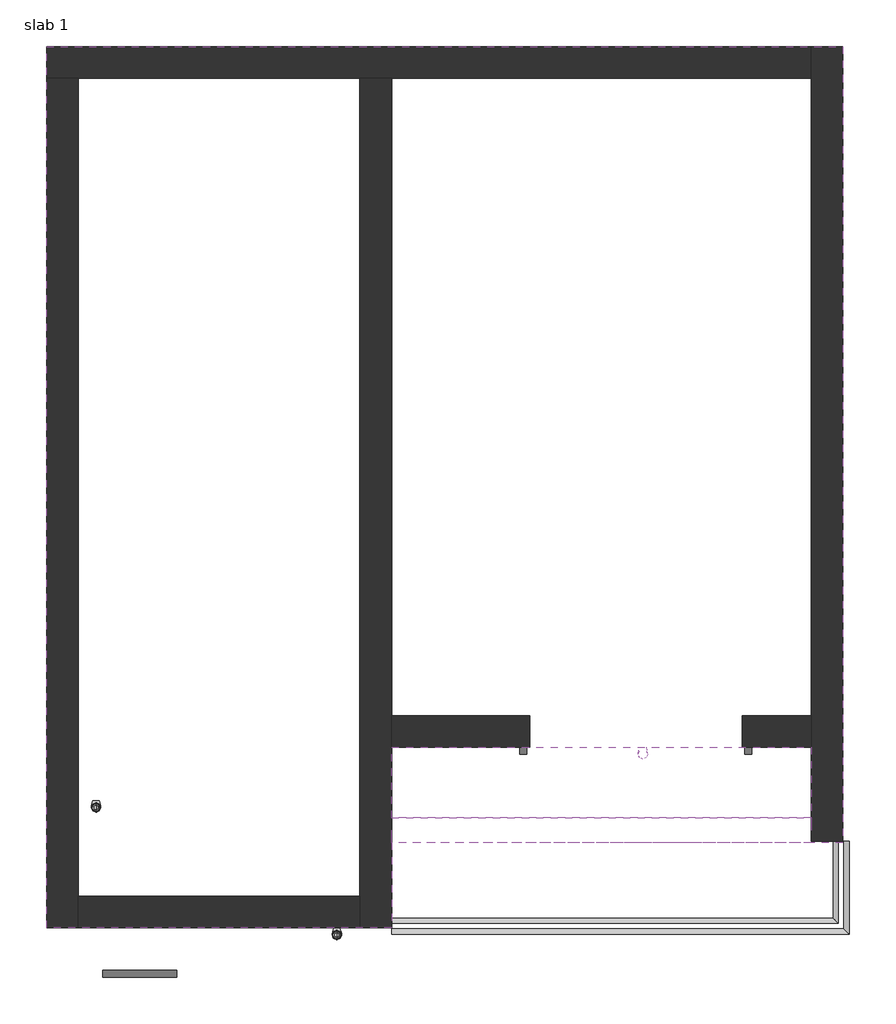
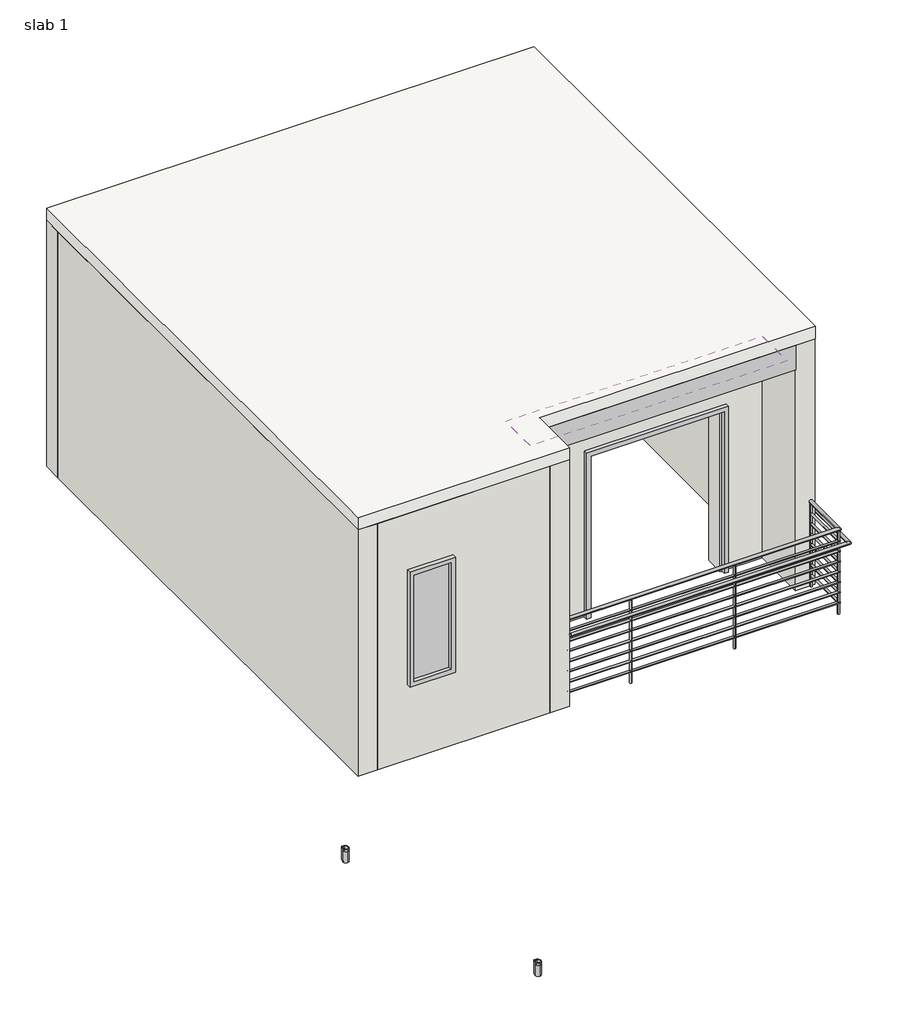
# One storey: 6 walls, 3 light fixtures, 3 proxies, 1 covering, 1 railing, 1 slab.
"""IFC4 building model written with IfcOpenShell, lengths in millimetres."""

from ifc_helpers import new_model, si_unit, point, frame, frame_2d, origin, place, context, project, spatial, polyline, circle_curve, ellipse_curve, trimmed, segment, composite_curve, outline, extrude, faceted_brep, transform, mapped, element, save
from ifc_brep_helpers import plane_surface, cylinder_surface, advanced_brep
from components import generic_models_1_generic_models_1_53319598, generic_models_3_generic_models_3_c6119d6a, generic_models_4_generic_models_4_090447d9, light_fixture_d13112ec

model = new_model("IFC4")

# Units and contexts
model_context = context("Model", 3, world=origin())
ifc_project = project(units=[si_unit("LENGTHUNIT", "METRE", prefix="MILLI")], contexts=[model_context])

# Site, building, storey
site = spatial("IfcSite", under=ifc_project)
building = spatial("IfcBuilding", under=site)
storey = spatial("IfcBuildingStorey", under=building, Name="slab 1", Elevation=3200.4)

# Proxies
placement = place(None, origin())
generic_models_1_generic_models_1_shape = generic_models_1_generic_models_1_53319598(model_context)
element("IfcBuildingElementProxy", 1, Name="Generic Models 1 : Generic Models 1", ObjectType="Generic Models 1 : Generic Models 1", at=placement, inside=storey, context=model_context, shape_type="MappedRepresentation", body=[
    mapped(generic_models_1_generic_models_1_shape, transform((0.0, 0.0, 0.0), x_axis=(1.0, 0.0, 0.0), y_axis=(0.0, 1.0, 0.0), z_axis=(0.0, 0.0, 1.0))),
])
generic_models_3_generic_models_3_shape = generic_models_3_generic_models_3_c6119d6a(model_context)
element("IfcBuildingElementProxy", 2, Name="Generic Models 3 : Generic Models 3", ObjectType="Generic Models 3 : Generic Models 3", at=placement, inside=storey, context=model_context, shape_type="MappedRepresentation", body=[
    mapped(generic_models_3_generic_models_3_shape, transform((0.0, 0.0, 0.0), x_axis=(1.0, 0.0, 0.0), y_axis=(0.0, 1.0, 0.0), z_axis=(0.0, 0.0, 1.0))),
])
generic_models_4_generic_models_4_shape = generic_models_4_generic_models_4_090447d9(model_context)
element("IfcBuildingElementProxy", 3, Name="Generic Models 4 : Generic Models 4", ObjectType="Generic Models 4 : Generic Models 4", at=placement, inside=storey, context=model_context, shape_type="MappedRepresentation", body=[
    mapped(generic_models_4_generic_models_4_shape, transform((0.0, 0.0, 0.0), x_axis=(1.0, 0.0, 0.0), y_axis=(0.0, 1.0, 0.0), z_axis=(0.0, 0.0, 1.0))),
])

# Covering
element("IfcCovering", 4, ObjectType="2' x 4' ACT System", at=placement, inside=storey, context=model_context, shape_type="SweptSolid", body=[
    extrude(outline(polyline([(-4601.1678816, 2126.5115792), (-7611.0678816, 2126.5115792), (-7611.0678816, 2631.9030358), (-4601.1678816, 2631.9030358), (-4601.1678816, 2126.5115792)])), frame((0.0, 0.0, 5943.6), z_axis=(0.0, 0.0, 1.0), x_axis=(1.0, 0.0, 0.0)), (0.0, 0.0, 1.0), 57.15),
])

# Light fixtures
light_fixture_shape = light_fixture_d13112ec(model_context)
element("IfcLightFixture", 5, at=placement, inside=storey, context=model_context, shape_type="MappedRepresentation", body=[
    mapped(light_fixture_shape, transform((-9731.9678816, 2250.9030358, 1580.2048365), x_axis=(1.0, 0.0, 0.0), y_axis=(0.0, 1.0, 0.0), z_axis=(0.0, 0.0, 1.0))),
])
element("IfcLightFixture", 6, at=placement, inside=storey, context=model_context, shape_type="MappedRepresentation", body=[
    mapped(light_fixture_shape, transform((-8004.7678816, 1336.5030358, 122.3083), x_axis=(1.0, 0.0, 0.0), y_axis=(0.0, 1.0, 0.0), z_axis=(0.0, 0.0, 1.0))),
])
element("IfcLightFixture", 7, at=placement, inside=storey, context=model_context, shape_type="MappedRepresentation", body=[
    mapped(light_fixture_shape, transform((-5808.000689, 2631.9030358, 5856.5439655), x_axis=(1.0, 0.0, 0.0), y_axis=(0.0, 1.0, 0.0), z_axis=(0.0, 0.0, 1.0))),
])

# Railing
element("IfcRailing", 8, ObjectType="Guardrail - Pipe", at=placement, inside=storey, context=model_context, shape_type="SolidModel", body=[
    advanced_brep(
    [(-4366.2178816, 1958.8030358, 4095.75), (-4328.1178816, 1958.8030358, 4095.75), (-4366.2178816, 1330.1530358, 4095.75), (-4328.1178816, 1292.0530358, 4095.75), (-7611.0678816, 1330.1530358, 4095.75), (-7611.0678816, 1292.0530358, 4095.75)],
    [
        (0, 1, circle_curve(frame((-4347.1678816, 1958.8030358, 4095.75), z_axis=(0.0, 1.0, 0.0), x_axis=(1.0, 0.0, 0.0)), 19.05)),
        (1, 0, circle_curve(frame((-4347.1678816, 1958.8030358, 4095.75), z_axis=(0.0, 1.0, 0.0), x_axis=(1.0, 0.0, 0.0)), 19.05)),
        (0, 2),
        (2, 3, ellipse_curve(frame((-4347.1678816, 1311.1030358, 4095.75), z_axis=(0.7071067811865487, 0.7071067811865464, 0.0), x_axis=(-0.7071067811865464, 0.7071067811865487, 0.0)), 26.9407684, 19.05)),
        (3, 1),
        (3, 2, ellipse_curve(frame((-4347.1678816, 1311.1030358, 4095.75), z_axis=(0.7071067811865487, 0.7071067811865464, 0.0), x_axis=(-0.7071067811865464, 0.7071067811865487, 0.0)), 26.9407684, 19.05)),
        (4, 5, circle_curve(frame((-7611.0678816, 1311.1030358, 4095.75), z_axis=(-1.0, 0.0, 0.0), x_axis=(0.0, -1.0, 0.0)), 19.05)),
        (5, 4, circle_curve(frame((-7611.0678816, 1311.1030358, 4095.75), z_axis=(-1.0, 0.0, 0.0), x_axis=(0.0, -1.0, 0.0)), 19.05)),
        (2, 4),
        (5, 3),
    ],
    [
        plane_surface(frame((-4347.1678816, 1958.8030358, 4114.8), z_axis=(0.0, 1.0, 0.0), x_axis=(0.0, 0.0, -1.0))),
        cylinder_surface(frame((-4347.1678816, 1958.8030358, 4095.75), z_axis=(0.0, 1.0, 0.0), x_axis=(1.0, 0.0, 0.0)), 19.05),
        plane_surface(frame((-7611.0678816, 1311.1030358, 4114.8), z_axis=(-1.0, 0.0, 0.0), x_axis=(0.0, -1.0, 0.0))),
        cylinder_surface(frame((-4347.1678816, 1311.1030358, 4095.75), z_axis=(1.0, 0.0, 0.0), x_axis=(0.0, -1.0, 0.0)), 19.05),
    ],
    [
        (0, [[1, 2]]),
        (1, [[-1, 3, 4, 5]]),
        (1, [[-2, -5, 6, -3]]),
        (2, [[7, 8]]),
        (3, [[-4, 9, -8, 10]]),
        (3, [[-6, -10, -7, -9]]),
    ],
),
    advanced_brep(
    [(-4442.4178816, 1958.8030358, 4248.15), (-4404.3178816, 1958.8030358, 4248.15), (-7611.0678816, 1406.3530358, 4248.15), (-7611.0678816, 1368.2530358, 4248.15), (-4442.4178816, 1406.3530358, 4248.15), (-4404.3178816, 1368.2530358, 4248.15)],
    [
        (0, 1, circle_curve(frame((-4423.3678816, 1958.8030358, 4248.15), z_axis=(0.0, 1.0, 0.0), x_axis=(1.0, 0.0, 0.0)), 19.05)),
        (1, 0, circle_curve(frame((-4423.3678816, 1958.8030358, 4248.15), z_axis=(0.0, 1.0, 0.0), x_axis=(1.0, 0.0, 0.0)), 19.05)),
        (2, 3, circle_curve(frame((-7611.0678816, 1387.3030358, 4248.15), z_axis=(-1.0, 0.0, 0.0), x_axis=(0.0, -1.0, 0.0)), 19.05)),
        (3, 2, circle_curve(frame((-7611.0678816, 1387.3030358, 4248.15), z_axis=(-1.0, 0.0, 0.0), x_axis=(0.0, -1.0, 0.0)), 19.05)),
        (0, 4),
        (4, 5, ellipse_curve(frame((-4423.3678816, 1387.3030358, 4248.15), z_axis=(0.7071067811865487, 0.7071067811865464, 0.0), x_axis=(-0.7071067811865464, 0.7071067811865487, 0.0)), 26.9407684, 19.05)),
        (5, 1),
        (5, 4, ellipse_curve(frame((-4423.3678816, 1387.3030358, 4248.15), z_axis=(0.7071067811865487, 0.7071067811865464, 0.0), x_axis=(-0.7071067811865464, 0.7071067811865487, 0.0)), 26.9407684, 19.05)),
        (4, 2),
        (3, 5),
    ],
    [
        plane_surface(frame((-4423.3678816, 1958.8030358, 4267.2), z_axis=(0.0, 1.0, 0.0), x_axis=(0.0, 0.0, -1.0))),
        plane_surface(frame((-7611.0678816, 1387.3030358, 4267.2), z_axis=(-1.0, 0.0, 0.0), x_axis=(0.0, -1.0, 0.0))),
        cylinder_surface(frame((-4423.3678816, 1958.8030358, 4248.15), z_axis=(0.0, 1.0, 0.0), x_axis=(1.0, 0.0, 0.0)), 19.05),
        cylinder_surface(frame((-4423.3678816, 1387.3030358, 4248.15), z_axis=(1.0, 0.0, 0.0), x_axis=(0.0, -1.0, 0.0)), 19.05),
    ],
    [
        (0, [[1, 2]]),
        (1, [[3, 4]]),
        (2, [[-1, 5, 6, 7]]),
        (2, [[-2, -7, 8, -5]]),
        (3, [[-6, 9, -4, 10]]),
        (3, [[-8, -10, -3, -9]]),
    ],
),
    advanced_brep(
    [(-4410.6678816, 1958.8030358, 4102.1), (-4436.0678816, 1958.8030358, 4102.1), (-7611.0678816, 1374.6030358, 4102.1), (-7611.0678816, 1400.0030358, 4102.1), (-4410.6678816, 1374.6030358, 4102.1), (-4436.0678816, 1400.0030358, 4102.1)],
    [
        (0, 1, circle_curve(frame((-4423.3678816, 1958.8030358, 4102.1), z_axis=(0.0, 1.0, 0.0), x_axis=(-1.0, 0.0, 0.0)), 12.7)),
        (1, 0, circle_curve(frame((-4423.3678816, 1958.8030358, 4102.1), z_axis=(0.0, 1.0, 0.0), x_axis=(-1.0, 0.0, 0.0)), 12.7)),
        (2, 3, circle_curve(frame((-7611.0678816, 1387.3030358, 4102.1), z_axis=(-1.0, 0.0, 0.0), x_axis=(0.0, 1.0, 0.0)), 12.7)),
        (3, 2, circle_curve(frame((-7611.0678816, 1387.3030358, 4102.1), z_axis=(-1.0, 0.0, 0.0), x_axis=(0.0, 1.0, 0.0)), 12.7)),
        (0, 4),
        (4, 5, ellipse_curve(frame((-4423.3678816, 1387.3030358, 4102.1), z_axis=(0.7071067811865487, 0.7071067811865464, 0.0), x_axis=(-0.7071067811865464, 0.7071067811865487, 0.0)), 17.9605122, 12.7)),
        (5, 1),
        (5, 4, ellipse_curve(frame((-4423.3678816, 1387.3030358, 4102.1), z_axis=(0.7071067811865487, 0.7071067811865464, 0.0), x_axis=(-0.7071067811865464, 0.7071067811865487, 0.0)), 17.9605122, 12.7)),
        (4, 2),
        (3, 5),
    ],
    [
        plane_surface(frame((-4423.3678816, 1958.8030358, 4114.8), z_axis=(0.0, 1.0, 0.0), x_axis=(0.0, 0.0, -1.0))),
        plane_surface(frame((-7611.0678816, 1387.3030358, 4114.8), z_axis=(-1.0, 0.0, 0.0), x_axis=(0.0, -1.0, 0.0))),
        cylinder_surface(frame((-4423.3678816, 1958.8030358, 4102.1), z_axis=(0.0, 1.0, 0.0), x_axis=(-1.0, 0.0, 0.0)), 12.7),
        cylinder_surface(frame((-4423.3678816, 1387.3030358, 4102.1), z_axis=(1.0, 0.0, 0.0), x_axis=(0.0, 1.0, 0.0)), 12.7),
    ],
    [
        (0, [[1, 2]]),
        (1, [[3, 4]]),
        (2, [[-1, 5, 6, 7]]),
        (2, [[-2, -7, 8, -5]]),
        (3, [[-6, 9, -4, 10]]),
        (3, [[-8, -10, -3, -9]]),
    ],
),
    advanced_brep(
    [(-4410.6678816, 1958.8030358, 3975.1), (-4436.0678816, 1958.8030358, 3975.1), (-7611.0678816, 1374.6030358, 3975.1), (-7611.0678816, 1400.0030358, 3975.1), (-4410.6678816, 1374.6030358, 3975.1), (-4436.0678816, 1400.0030358, 3975.1)],
    [
        (0, 1, circle_curve(frame((-4423.3678816, 1958.8030358, 3975.1), z_axis=(0.0, 1.0, 0.0), x_axis=(-1.0, 0.0, 0.0)), 12.7)),
        (1, 0, circle_curve(frame((-4423.3678816, 1958.8030358, 3975.1), z_axis=(0.0, 1.0, 0.0), x_axis=(-1.0, 0.0, 0.0)), 12.7)),
        (2, 3, circle_curve(frame((-7611.0678816, 1387.3030358, 3975.1), z_axis=(-1.0, 0.0, 0.0), x_axis=(0.0, 1.0, 0.0)), 12.7)),
        (3, 2, circle_curve(frame((-7611.0678816, 1387.3030358, 3975.1), z_axis=(-1.0, 0.0, 0.0), x_axis=(0.0, 1.0, 0.0)), 12.7)),
        (0, 4),
        (4, 5, ellipse_curve(frame((-4423.3678816, 1387.3030358, 3975.1), z_axis=(0.7071067811865487, 0.7071067811865464, 0.0), x_axis=(-0.7071067811865464, 0.7071067811865487, 0.0)), 17.9605122, 12.7)),
        (5, 1),
        (5, 4, ellipse_curve(frame((-4423.3678816, 1387.3030358, 3975.1), z_axis=(0.7071067811865487, 0.7071067811865464, 0.0), x_axis=(-0.7071067811865464, 0.7071067811865487, 0.0)), 17.9605122, 12.7)),
        (4, 2),
        (3, 5),
    ],
    [
        plane_surface(frame((-4423.3678816, 1958.8030358, 3987.8), z_axis=(0.0, 1.0, 0.0), x_axis=(0.0, 0.0, -1.0))),
        plane_surface(frame((-7611.0678816, 1387.3030358, 3987.8), z_axis=(-1.0, 0.0, 0.0), x_axis=(0.0, -1.0, 0.0))),
        cylinder_surface(frame((-4423.3678816, 1958.8030358, 3975.1), z_axis=(0.0, 1.0, 0.0), x_axis=(-1.0, 0.0, 0.0)), 12.7),
        cylinder_surface(frame((-4423.3678816, 1387.3030358, 3975.1), z_axis=(1.0, 0.0, 0.0), x_axis=(0.0, 1.0, 0.0)), 12.7),
    ],
    [
        (0, [[1, 2]]),
        (1, [[3, 4]]),
        (2, [[-1, 5, 6, 7]]),
        (2, [[-2, -7, 8, -5]]),
        (3, [[-6, 9, -4, 10]]),
        (3, [[-8, -10, -3, -9]]),
    ],
),
    advanced_brep(
    [(-4410.6678816, 1958.8030358, 3848.1), (-4436.0678816, 1958.8030358, 3848.1), (-4410.6678816, 1374.6030358, 3848.1), (-4436.0678816, 1400.0030358, 3848.1), (-7611.0678816, 1374.6030358, 3848.1), (-7611.0678816, 1400.0030358, 3848.1)],
    [
        (0, 1, circle_curve(frame((-4423.3678816, 1958.8030358, 3848.1), z_axis=(0.0, 1.0, 0.0), x_axis=(-1.0, 0.0, 0.0)), 12.7)),
        (1, 0, circle_curve(frame((-4423.3678816, 1958.8030358, 3848.1), z_axis=(0.0, 1.0, 0.0), x_axis=(-1.0, 0.0, 0.0)), 12.7)),
        (0, 2),
        (2, 3, ellipse_curve(frame((-4423.3678816, 1387.3030358, 3848.1), z_axis=(0.7071067811865487, 0.7071067811865464, 0.0), x_axis=(-0.7071067811865464, 0.7071067811865487, 0.0)), 17.9605122, 12.7)),
        (3, 1),
        (3, 2, ellipse_curve(frame((-4423.3678816, 1387.3030358, 3848.1), z_axis=(0.7071067811865487, 0.7071067811865464, 0.0), x_axis=(-0.7071067811865464, 0.7071067811865487, 0.0)), 17.9605122, 12.7)),
        (4, 5, circle_curve(frame((-7611.0678816, 1387.3030358, 3848.1), z_axis=(-1.0, 0.0, 0.0), x_axis=(0.0, 1.0, 0.0)), 12.7)),
        (5, 4, circle_curve(frame((-7611.0678816, 1387.3030358, 3848.1), z_axis=(-1.0, 0.0, 0.0), x_axis=(0.0, 1.0, 0.0)), 12.7)),
        (2, 4),
        (5, 3),
    ],
    [
        plane_surface(frame((-4423.3678816, 1958.8030358, 3860.8), z_axis=(0.0, 1.0, 0.0), x_axis=(0.0, 0.0, -1.0))),
        cylinder_surface(frame((-4423.3678816, 1958.8030358, 3848.1), z_axis=(0.0, 1.0, 0.0), x_axis=(-1.0, 0.0, 0.0)), 12.7),
        plane_surface(frame((-7611.0678816, 1387.3030358, 3860.8), z_axis=(-1.0, 0.0, 0.0), x_axis=(0.0, -1.0, 0.0))),
        cylinder_surface(frame((-4423.3678816, 1387.3030358, 3848.1), z_axis=(1.0, 0.0, 0.0), x_axis=(0.0, 1.0, 0.0)), 12.7),
    ],
    [
        (0, [[1, 2]]),
        (1, [[-1, 3, 4, 5]]),
        (1, [[-2, -5, 6, -3]]),
        (2, [[7, 8]]),
        (3, [[-4, 9, -8, 10]]),
        (3, [[-6, -10, -7, -9]]),
    ],
),
    advanced_brep(
    [(-4410.6678816, 1958.8030358, 3721.1), (-4436.0678816, 1958.8030358, 3721.1), (-4410.6678816, 1374.6030358, 3721.1), (-4436.0678816, 1400.0030358, 3721.1), (-7611.0678816, 1374.6030358, 3721.1), (-7611.0678816, 1400.0030358, 3721.1)],
    [
        (0, 1, circle_curve(frame((-4423.3678816, 1958.8030358, 3721.1), z_axis=(0.0, 1.0, 0.0), x_axis=(-1.0, 0.0, 0.0)), 12.7)),
        (1, 0, circle_curve(frame((-4423.3678816, 1958.8030358, 3721.1), z_axis=(0.0, 1.0, 0.0), x_axis=(-1.0, 0.0, 0.0)), 12.7)),
        (0, 2),
        (2, 3, ellipse_curve(frame((-4423.3678816, 1387.3030358, 3721.1), z_axis=(0.7071067811865487, 0.7071067811865464, 0.0), x_axis=(-0.7071067811865464, 0.7071067811865487, 0.0)), 17.9605122, 12.7)),
        (3, 1),
        (3, 2, ellipse_curve(frame((-4423.3678816, 1387.3030358, 3721.1), z_axis=(0.7071067811865487, 0.7071067811865464, 0.0), x_axis=(-0.7071067811865464, 0.7071067811865487, 0.0)), 17.9605122, 12.7)),
        (4, 5, circle_curve(frame((-7611.0678816, 1387.3030358, 3721.1), z_axis=(-1.0, 0.0, 0.0), x_axis=(0.0, 1.0, 0.0)), 12.7)),
        (5, 4, circle_curve(frame((-7611.0678816, 1387.3030358, 3721.1), z_axis=(-1.0, 0.0, 0.0), x_axis=(0.0, 1.0, 0.0)), 12.7)),
        (2, 4),
        (5, 3),
    ],
    [
        plane_surface(frame((-4423.3678816, 1958.8030358, 3733.8), z_axis=(0.0, 1.0, 0.0), x_axis=(0.0, 0.0, -1.0))),
        cylinder_surface(frame((-4423.3678816, 1958.8030358, 3721.1), z_axis=(0.0, 1.0, 0.0), x_axis=(-1.0, 0.0, 0.0)), 12.7),
        plane_surface(frame((-7611.0678816, 1387.3030358, 3733.8), z_axis=(-1.0, 0.0, 0.0), x_axis=(0.0, -1.0, 0.0))),
        cylinder_surface(frame((-4423.3678816, 1387.3030358, 3721.1), z_axis=(1.0, 0.0, 0.0), x_axis=(0.0, 1.0, 0.0)), 12.7),
    ],
    [
        (0, [[1, 2]]),
        (1, [[-1, 3, 4, 5]]),
        (1, [[-2, -5, 6, -3]]),
        (2, [[7, 8]]),
        (3, [[-4, 9, -8, 10]]),
        (3, [[-6, -10, -7, -9]]),
    ],
),
    advanced_brep(
    [(-4410.6678816, 1958.8030358, 3594.1), (-4436.0678816, 1958.8030358, 3594.1), (-4410.6678816, 1374.6030358, 3594.1), (-4436.0678816, 1400.0030358, 3594.1), (-7611.0678816, 1374.6030358, 3594.1), (-7611.0678816, 1400.0030358, 3594.1)],
    [
        (0, 1, circle_curve(frame((-4423.3678816, 1958.8030358, 3594.1), z_axis=(0.0, 1.0, 0.0), x_axis=(-1.0, 0.0, 0.0)), 12.7)),
        (1, 0, circle_curve(frame((-4423.3678816, 1958.8030358, 3594.1), z_axis=(0.0, 1.0, 0.0), x_axis=(-1.0, 0.0, 0.0)), 12.7)),
        (0, 2),
        (2, 3, ellipse_curve(frame((-4423.3678816, 1387.3030358, 3594.1), z_axis=(0.7071067811865487, 0.7071067811865464, 0.0), x_axis=(-0.7071067811865464, 0.7071067811865487, 0.0)), 17.9605122, 12.7)),
        (3, 1),
        (3, 2, ellipse_curve(frame((-4423.3678816, 1387.3030358, 3594.1), z_axis=(0.7071067811865487, 0.7071067811865464, 0.0), x_axis=(-0.7071067811865464, 0.7071067811865487, 0.0)), 17.9605122, 12.7)),
        (4, 5, circle_curve(frame((-7611.0678816, 1387.3030358, 3594.1), z_axis=(-1.0, 0.0, 0.0), x_axis=(0.0, 1.0, 0.0)), 12.7)),
        (5, 4, circle_curve(frame((-7611.0678816, 1387.3030358, 3594.1), z_axis=(-1.0, 0.0, 0.0), x_axis=(0.0, 1.0, 0.0)), 12.7)),
        (2, 4),
        (5, 3),
    ],
    [
        plane_surface(frame((-4423.3678816, 1958.8030358, 3606.8), z_axis=(0.0, 1.0, 0.0), x_axis=(0.0, 0.0, -1.0))),
        cylinder_surface(frame((-4423.3678816, 1958.8030358, 3594.1), z_axis=(0.0, 1.0, 0.0), x_axis=(-1.0, 0.0, 0.0)), 12.7),
        plane_surface(frame((-7611.0678816, 1387.3030358, 3606.8), z_axis=(-1.0, 0.0, 0.0), x_axis=(0.0, -1.0, 0.0))),
        cylinder_surface(frame((-4423.3678816, 1387.3030358, 3594.1), z_axis=(1.0, 0.0, 0.0), x_axis=(0.0, 1.0, 0.0)), 12.7),
    ],
    [
        (0, [[1, 2]]),
        (1, [[-1, 3, 4, 5]]),
        (1, [[-2, -5, 6, -3]]),
        (2, [[7, 8]]),
        (3, [[-4, 9, -8, 10]]),
        (3, [[-6, -10, -7, -9]]),
    ],
),
    advanced_brep(
    [(-4410.6678816, 1958.8030358, 3467.1), (-4436.0678816, 1958.8030358, 3467.1), (-4410.6678816, 1374.6030358, 3467.1), (-4436.0678816, 1400.0030358, 3467.1), (-7611.0678816, 1374.6030358, 3467.1), (-7611.0678816, 1400.0030358, 3467.1)],
    [
        (0, 1, circle_curve(frame((-4423.3678816, 1958.8030358, 3467.1), z_axis=(0.0, 1.0, 0.0), x_axis=(-1.0, 0.0, 0.0)), 12.7)),
        (1, 0, circle_curve(frame((-4423.3678816, 1958.8030358, 3467.1), z_axis=(0.0, 1.0, 0.0), x_axis=(-1.0, 0.0, 0.0)), 12.7)),
        (0, 2),
        (2, 3, ellipse_curve(frame((-4423.3678816, 1387.3030358, 3467.1), z_axis=(0.7071067811865487, 0.7071067811865464, 0.0), x_axis=(-0.7071067811865464, 0.7071067811865487, 0.0)), 17.9605122, 12.7)),
        (3, 1),
        (3, 2, ellipse_curve(frame((-4423.3678816, 1387.3030358, 3467.1), z_axis=(0.7071067811865487, 0.7071067811865464, 0.0), x_axis=(-0.7071067811865464, 0.7071067811865487, 0.0)), 17.9605122, 12.7)),
        (4, 5, circle_curve(frame((-7611.0678816, 1387.3030358, 3467.1), z_axis=(-1.0, 0.0, 0.0), x_axis=(0.0, 1.0, 0.0)), 12.7)),
        (5, 4, circle_curve(frame((-7611.0678816, 1387.3030358, 3467.1), z_axis=(-1.0, 0.0, 0.0), x_axis=(0.0, 1.0, 0.0)), 12.7)),
        (2, 4),
        (5, 3),
    ],
    [
        plane_surface(frame((-4423.3678816, 1958.8030358, 3479.8), z_axis=(0.0, 1.0, 0.0), x_axis=(0.0, 0.0, -1.0))),
        cylinder_surface(frame((-4423.3678816, 1958.8030358, 3467.1), z_axis=(0.0, 1.0, 0.0), x_axis=(-1.0, 0.0, 0.0)), 12.7),
        plane_surface(frame((-7611.0678816, 1387.3030358, 3479.8), z_axis=(-1.0, 0.0, 0.0), x_axis=(0.0, -1.0, 0.0))),
        cylinder_surface(frame((-4423.3678816, 1387.3030358, 3467.1), z_axis=(1.0, 0.0, 0.0), x_axis=(0.0, 1.0, 0.0)), 12.7),
    ],
    [
        (0, [[1, 2]]),
        (1, [[-1, 3, 4, 5]]),
        (1, [[-2, -5, 6, -3]]),
        (2, [[7, 8]]),
        (3, [[-4, 9, -8, 10]]),
        (3, [[-6, -10, -7, -9]]),
    ],
),
    advanced_brep(
    [(-4410.6678816, 1958.8030358, 3340.1), (-4436.0678816, 1958.8030358, 3340.1), (-4410.6678816, 1374.6030358, 3340.1), (-4436.0678816, 1400.0030358, 3340.1), (-7611.0678816, 1374.6030358, 3340.1), (-7611.0678816, 1400.0030358, 3340.1)],
    [
        (0, 1, circle_curve(frame((-4423.3678816, 1958.8030358, 3340.1), z_axis=(0.0, 1.0, 0.0), x_axis=(-1.0, 0.0, 0.0)), 12.7)),
        (1, 0, circle_curve(frame((-4423.3678816, 1958.8030358, 3340.1), z_axis=(0.0, 1.0, 0.0), x_axis=(-1.0, 0.0, 0.0)), 12.7)),
        (0, 2),
        (2, 3, ellipse_curve(frame((-4423.3678816, 1387.3030358, 3340.1), z_axis=(0.7071067811865487, 0.7071067811865464, 0.0), x_axis=(-0.7071067811865464, 0.7071067811865487, 0.0)), 17.9605122, 12.7)),
        (3, 1),
        (3, 2, ellipse_curve(frame((-4423.3678816, 1387.3030358, 3340.1), z_axis=(0.7071067811865487, 0.7071067811865464, 0.0), x_axis=(-0.7071067811865464, 0.7071067811865487, 0.0)), 17.9605122, 12.7)),
        (4, 5, circle_curve(frame((-7611.0678816, 1387.3030358, 3340.1), z_axis=(-1.0, 0.0, 0.0), x_axis=(0.0, 1.0, 0.0)), 12.7)),
        (5, 4, circle_curve(frame((-7611.0678816, 1387.3030358, 3340.1), z_axis=(-1.0, 0.0, 0.0), x_axis=(0.0, 1.0, 0.0)), 12.7)),
        (2, 4),
        (5, 3),
    ],
    [
        plane_surface(frame((-4423.3678816, 1958.8030358, 3352.8), z_axis=(0.0, 1.0, 0.0), x_axis=(0.0, 0.0, -1.0))),
        cylinder_surface(frame((-4423.3678816, 1958.8030358, 3340.1), z_axis=(0.0, 1.0, 0.0), x_axis=(-1.0, 0.0, 0.0)), 12.7),
        plane_surface(frame((-7611.0678816, 1387.3030358, 3352.8), z_axis=(-1.0, 0.0, 0.0), x_axis=(0.0, -1.0, 0.0))),
        cylinder_surface(frame((-4423.3678816, 1387.3030358, 3340.1), z_axis=(1.0, 0.0, 0.0), x_axis=(0.0, 1.0, 0.0)), 12.7),
    ],
    [
        (0, [[1, 2]]),
        (1, [[-1, 3, 4, 5]]),
        (1, [[-2, -5, 6, -3]]),
        (2, [[7, 8]]),
        (3, [[-4, 9, -8, 10]]),
        (3, [[-6, -10, -7, -9]]),
    ],
),
    extrude(outline(composite_curve([segment(trimmed(circle_curve(frame_2d((-6861.7678816, 1387.3030358)), 12.7), [point((-6861.7678816, 1374.6030358))], [point((-6861.7678816, 1400.0030358))], False, "CARTESIAN"), True, "CONTINUOUS"), segment(trimmed(circle_curve(frame_2d((-6861.7678816, 1387.3030358)), 12.7), [point((-6861.7678816, 1400.0030358))], [point((-6861.7678816, 1374.6030358))], False, "CARTESIAN"), True, "CONTINUOUS")], self_intersect=False)), frame((0.0, 0.0, 3200.4), z_axis=(0.0, 0.0, 1.0), x_axis=(1.0, 0.0, 0.0)), (0.0, 0.0, 1.0), 1028.7),
    extrude(outline(composite_curve([segment(trimmed(circle_curve(frame_2d((-5642.5678816, 1387.3030358)), 12.7), [point((-5642.5678816, 1374.6030358))], [point((-5642.5678816, 1400.0030358))], False, "CARTESIAN"), True, "CONTINUOUS"), segment(trimmed(circle_curve(frame_2d((-5642.5678816, 1387.3030358)), 12.7), [point((-5642.5678816, 1400.0030358))], [point((-5642.5678816, 1374.6030358))], False, "CARTESIAN"), True, "CONTINUOUS")], self_intersect=False)), frame((0.0, 0.0, 3200.4), z_axis=(0.0, 0.0, 1.0), x_axis=(1.0, 0.0, 0.0)), (0.0, 0.0, 1.0), 1028.7),
    extrude(outline(composite_curve([segment(trimmed(circle_curve(frame_2d((-4423.3678816, 1387.3030358)), 12.7), [point((-4410.6678816, 1387.3030358))], [point((-4436.0678816, 1387.3030358))], False, "CARTESIAN"), True, "CONTINUOUS"), segment(trimmed(circle_curve(frame_2d((-4423.3678816, 1387.3030358)), 12.7), [point((-4436.0678816, 1387.3030358))], [point((-4410.6678816, 1387.3030358))], False, "CARTESIAN"), True, "CONTINUOUS")], self_intersect=False)), frame((0.0, 0.0, 3200.4), z_axis=(0.0, 0.0, 1.0), x_axis=(1.0, 0.0, 0.0)), (0.0, 0.0, 1.0), 1028.7),
    extrude(outline(composite_curve([segment(trimmed(circle_curve(frame_2d((-7598.3678816, 1387.3030358)), 12.7), [point((-7598.3678816, 1374.6030358))], [point((-7598.3678816, 1400.0030358))], False, "CARTESIAN"), True, "CONTINUOUS"), segment(trimmed(circle_curve(frame_2d((-7598.3678816, 1387.3030358)), 12.7), [point((-7598.3678816, 1400.0030358))], [point((-7598.3678816, 1374.6030358))], False, "CARTESIAN"), True, "CONTINUOUS")], self_intersect=False)), frame((0.0, 0.0, 3200.4), z_axis=(0.0, 0.0, 1.0), x_axis=(1.0, 0.0, 0.0)), (0.0, 0.0, 1.0), 1028.7),
    extrude(outline(composite_curve([segment(trimmed(circle_curve(frame_2d((-4423.3678816, 1946.1030358)), 12.7), [point((-4410.6678816, 1946.1030358))], [point((-4436.0678816, 1946.1030358))], False, "CARTESIAN"), True, "CONTINUOUS"), segment(trimmed(circle_curve(frame_2d((-4423.3678816, 1946.1030358)), 12.7), [point((-4436.0678816, 1946.1030358))], [point((-4410.6678816, 1946.1030358))], False, "CARTESIAN"), True, "CONTINUOUS")], self_intersect=False)), frame((0.0, 0.0, 3200.4), z_axis=(0.0, 0.0, 1.0), x_axis=(1.0, 0.0, 0.0)), (0.0, 0.0, 1.0), 1028.7),
])

# Slab
element("IfcSlab", 9, ObjectType="Generic - 6\"", at=placement, inside=storey, context=model_context, shape_type="SweptSolid", body=[
    extrude(outline(polyline([(-7611.0678816, 1336.5030358), (-10087.5678816, 1336.5030358), (-10087.5678816, 7661.1030358), (-4372.5678816, 7661.1030358), (-4372.5678816, 1946.1030358), (-7611.0678816, 1946.1030358), (-7611.0678816, 1336.5030358)])), frame((0.0, 0.0, 6248.4), z_axis=(0.0, 0.0, 1.0), x_axis=(1.0, 0.0, 0.0)), (0.0, 0.0, 1.0), 152.4),
])

# Walls
element("IfcWall", 10, ObjectType="Generic - 9\"", at=placement, inside=storey, context=model_context, shape_type="Brep", body=[
    faceted_brep([(-4601.1678816, 7661.1030358, 3200.4), (-4601.1678816, 7432.5030358, 3200.4), (-4601.1678816, 2860.5030358, 3200.4), (-4601.1678816, 2631.9030358, 3200.4), (-4601.1678816, 1958.8030358, 3200.4), (-4601.1678816, 1958.8030358, 6248.4), (-4601.1678816, 2631.9030358, 6248.4), (-4601.1678816, 2860.5030358, 6248.4), (-4601.1678816, 7432.5030358, 6248.4), (-4601.1678816, 7661.1030358, 6248.4), (-4372.5678816, 7661.1030358, 3200.4), (-4372.5678816, 7661.1030358, 6248.4), (-4372.5678816, 1958.8030358, 6248.4), (-4372.5678816, 1958.8030358, 3200.4)], [[[0, 1, 2, 3, 4, 5, 6, 7, 8, 9]], [[10, 11, 12, 13]], [[4, 3, 2, 1, 0, 10, 13]], [[5, 4, 13, 12]], [[9, 8, 7, 6, 5, 12, 11]], [[0, 9, 11, 10]]]),
])
element("IfcWall", 11, ObjectType="Generic - 9\"", at=placement, inside=storey, context=model_context, shape_type="Brep", body=[
    faceted_brep([(-10087.5678816, 7432.5030358, 3200.4), (-9858.9678816, 7432.5030358, 3200.4), (-7839.6678816, 7432.5030358, 3200.4), (-7611.0678816, 7432.5030358, 3200.4), (-4601.1678816, 7432.5030358, 3200.4), (-4601.1678816, 7432.5030358, 6248.4), (-7611.0678816, 7432.5030358, 6248.4), (-7839.6678816, 7432.5030358, 6248.4), (-9858.9678816, 7432.5030358, 6248.4), (-10087.5678816, 7432.5030358, 6248.4), (-10087.5678816, 7661.1030358, 3200.4), (-10087.5678816, 7661.1030358, 6248.4), (-4601.1678816, 7661.1030358, 6248.4), (-4601.1678816, 7661.1030358, 3200.4)], [[[0, 1, 2, 3, 4, 5, 6, 7, 8, 9]], [[10, 11, 12, 13]], [[4, 3, 2, 1, 0, 10, 13]], [[9, 8, 7, 6, 5, 12, 11]], [[5, 4, 13, 12]], [[0, 9, 11, 10]]]),
])
element("IfcWall", 12, ObjectType="Generic - 9\"", at=placement, inside=storey, context=model_context, shape_type="Brep", body=[
    faceted_brep([(-9858.9678816, 1336.5030358, 3200.4), (-9858.9678816, 1565.1030358, 3200.4), (-9858.9678816, 7432.5030358, 3200.4), (-9858.9678816, 7432.5030358, 6248.4), (-9858.9678816, 1565.1030358, 6248.4), (-9858.9678816, 1336.5030358, 6248.4), (-10087.5678816, 1336.5030358, 3200.4), (-10087.5678816, 1336.5030358, 6248.4), (-10087.5678816, 7432.5030358, 6248.4), (-10087.5678816, 7432.5030358, 3200.4)], [[[0, 1, 2, 3, 4, 5]], [[6, 7, 8, 9]], [[2, 1, 0, 6, 9]], [[5, 4, 3, 8, 7]], [[3, 2, 9, 8]], [[0, 5, 7, 6]]]),
])
element("IfcWall", 13, ObjectType="Generic - 9\"", at=placement, inside=storey, context=model_context, shape_type="Brep", body=[
    faceted_brep([(-7611.0678816, 1336.5030358, 3200.4), (-7611.0678816, 2631.9030358, 3200.4), (-7611.0678816, 2860.5030358, 3200.4), (-7611.0678816, 7432.5030358, 3200.4), (-7611.0678816, 7432.5030358, 6248.4), (-7611.0678816, 2860.5030358, 6248.4), (-7611.0678816, 2631.9030358, 6248.4), (-7611.0678816, 1336.5030358, 6248.4), (-7839.6678816, 1336.5030358, 3200.4), (-7839.6678816, 1336.5030358, 6248.4), (-7839.6678816, 1565.1030358, 6248.4), (-7839.6678816, 7432.5030358, 6248.4), (-7839.6678816, 7432.5030358, 3200.4), (-7839.6678816, 1565.1030358, 3200.4)], [[[0, 1, 2, 3, 4, 5, 6, 7]], [[8, 9, 10, 11, 12, 13]], [[3, 2, 1, 0, 8, 13, 12]], [[7, 6, 5, 4, 11, 10, 9]], [[4, 3, 12, 11]], [[0, 7, 9, 8]]]),
])
element("IfcWall", 14, ObjectType="Generic - 9\"", at=placement, inside=storey, context=model_context, shape_type="SweptSolid", body=[
    extrude(outline(polyline([(-7839.6678816, 1336.5030358), (-9858.9678816, 1336.5030358), (-9858.9678816, 1565.1030358), (-7839.6678816, 1565.1030358), (-7839.6678816, 1336.5030358)])), frame((0.0, 0.0, 3200.4), z_axis=(0.0, 0.0, 1.0), x_axis=(1.0, 0.0, 0.0)), (0.0, 0.0, 1.0), 3048.0),
])
element("IfcWall", 15, ObjectType="Generic - 9\"", at=placement, inside=storey, context=model_context, shape_type="SweptSolid", body=[
    extrude(outline(polyline([(6248.4, -4601.1678816), (6248.4, -7611.0678816), (3200.4, -7611.0678816), (3200.4, -6620.4678816), (5181.6, -6620.4678816), (5181.6, -5096.4678816), (3200.4, -5096.4678816), (3200.4, -4601.1678816), (6248.4, -4601.1678816)])), frame((0.0, 2631.9030358, 0.0), z_axis=(0.0, 1.0, 0.0), x_axis=(0.0, 0.0, 1.0)), (0.0, 0.0, 1.0), 228.6),
])

save(model, "model.ifc")

# Revit data of these elements
# Type "2' x 4' ACT System"
#   Assembly Code = "C3030210"
#   built-in parameter 1002203 = 1 (stored number, unit not read)
#   built-in parameter 1002202 = 1 (stored number, unit not read)
#   Layers, outside or top first: 0' - 1 5/8" "Default" (function 1); 0' - 0 5/8" "Acoustic Ceiling Tile 24 x 48" (function 5)
# Type
#   URL = "https://products-archive.xal.com/product/xal/048-31604111O"
#   Type Tag = ""
#   System = ""
#   Sorting Reference = ""
#   Schedule ID = "1"
#   Product Info = "SASSO 60 round direct / indirect wall | jet black | 2700 K | non DIM | UGR ?  22 | 1170 lm"
#   Photometric Web File = "XAL-OPAL-LAMBERTSCH_F16_AD62946.ies"
#   Optic = "opal (lambertsch)"
#   Manufacturer = "XAL"
#   Luminous Flux = "1170"
#   Item Number = "048-31604111O"
#   Initial Color Temperature = "2700 K"
#   Housing Color = "black/black"
#   Glare Rating = "22"
#   Description = "Cylindrical wall surface mounted luminaire made of aluminium; surface jet black powder coated;  passive cooling of the LEDs through improved heat sink geometry; with COB (Chip on Board) technology for maximum efficiency; no appearance of multiple shadows; light color 2700 K;  energy efficient LEDs with high CRI; incl. high quality lens system; homogeneous wall or ceiling illumination through uniform light distribution; direct/indirect light distribution;    incl. converter, non dimmable;  \r\nGeneral: jet black, 1170 lm\r\nLED: 2700 K\r\nOptical: opal (lambertsch), UGR ? 22\r\nElectrical: non DIM,  system 20.6 W\r\nPhysical: length 68 mm, width 84 mm, height 166 mm"
#   Control = "non DIM"
#   Color Temperature = "2700 K"
#   Catalog Number = "048-31604111O"
#   Assembly ID [instance] = ""
#   Additional Reference [instance] = ""
#   W = 0' - 3.30709"
#   Type Tag Object Distance [instance] = 0' - 0"
#   Type Tag Distance [instance] = 0' - 9.84252"
#   Type Tag Base Position [instance] = 0' - 9.84252"
#   Power = 20.6 W
#   L = 0' - 2.67717"
#   H = 0' - 6.53543"
#   Emit from Width = 1' - 3.74803"
#   Emit from Length = 0' - 3.93701"
#   Emit from Diameter = 0' - 2.16535"
#   Default Elevation = 4' - 0"
#   Type Tag Upper Position [instance] = no
#   Type Tag On [instance] = no
#   Type Tag Lower Position [instance] = yes
#   Tag Frame [instance] = no
#   Pcs. per Package = 1
#   Tag Size = element 383008
#   Product Color Secondary = XAL_JET_BLACK
#   Product Color Primary = XAL_JET_BLACK
#   Light type = element 382996
# Type "Guardrail - Pipe"
#   Assembly Code = "C2010400"
#   built-in parameter 1008612 = 0.0416667 (stored number, unit not read)
#   built-in parameter 1008611 = 0.0833333 (stored number, unit not read)
#   built-in parameter 1008609 = 4 (stored number, unit not read)
#   built-in parameter 1008604 = 0.166667 (stored number, unit not read)
#   built-in parameter 1008603 = 0.166667 (stored number, unit not read)
#   Railing Height = 3' - 6"
#   built-in parameter 1008630 = 2
#   built-in parameter 1008610 = 1
#   built-in parameter 1008605 = 1
#   built-in parameter 1008618 = Baluster - Round : 1"
# Type "Generic - 6\""
#   Assembly Code = "B1010"
#   Function = 0
#   Layers, outside or top first: 0' - 6" no material (function 1)
# Type "Generic - 9\""
#   Assembly Code = "B2010"
#   Layers, outside or top first: 0' - 9" no material (function 1)
# Element 1 (IfcBuildingElementProxy, "Generic Models 1 : Generic Models 1")
#   Phase Created = New Construction
#   Materials on its faces: "wall paint"
# Element 2 (IfcBuildingElementProxy, "Generic Models 3 : Generic Models 3")
#   Phase Created = New Construction
#   Materials on its faces: "Damp-proofing"
# Element 3 (IfcBuildingElementProxy, "Generic Models 4 : Generic Models 4")
#   Phase Created = New Construction
#   Materials on its faces: "Damp-proofing"
# Element 4 (IfcCovering, "2' x 4' ACT System")
#   Height Offset From Level = 9' - 0"
#   Phase Created = New Construction
#   Materials on its faces: "Acoustic Ceiling Tile 24 x 48", "Default", "wall paint"
# Element 5 (IfcLightFixture)
#   Mark = "1"
#   Assembly ID = ""
#   Additional Reference = ""
#   Type Tag Object Distance = 0' - 0"
#   Type Tag Distance = 0' - 9.84252"
#   Type Tag Base Position = 0' - 9.84252"
#   Type Tag Upper Position = no
#   Type Tag On = no
#   Type Tag Lower Position = yes
#   Tag Frame = no
#   Phase Created = New Construction
#   Materials on its faces: "XAL_JET_BLACK", "XAL_DIFFUSE"
# Element 6 (IfcLightFixture)
#   Mark = "2"
#   Assembly ID = ""
#   Additional Reference = ""
#   Type Tag Object Distance = 0' - 0"
#   Type Tag Distance = 0' - 9.84252"
#   Type Tag Base Position = 0' - 9.84252"
#   Type Tag Upper Position = no
#   Type Tag On = no
#   Type Tag Lower Position = yes
#   Tag Frame = no
#   Phase Created = New Construction
#   Materials on its faces: "XAL_JET_BLACK", "XAL_DIFFUSE"
# Element 7 (IfcLightFixture)
#   Mark = "3"
#   Assembly ID = ""
#   Additional Reference = ""
#   Type Tag Object Distance = 0' - 0"
#   Type Tag Distance = 0' - 9.84252"
#   Type Tag Base Position = 0' - 9.84252"
#   Type Tag Upper Position = no
#   Type Tag On = no
#   Type Tag Lower Position = yes
#   Tag Frame = no
#   Phase Created = New Construction
#   Materials on its faces: "XAL_JET_BLACK", "XAL_DIFFUSE"
# Element 8 (IfcRailing, "Guardrail - Pipe")
#   Phase Created = New Construction
# Element 9 (IfcSlab, "Generic - 6\"")
#   Height Offset From Level = 10' - 6"
#   Phase Created = New Construction
#   Materials on its faces: "Default Floor", "wall paint"
# Elements 10, 11, 12, 15 (IfcWall, "Generic - 9\"")
#   Top Offset = 0' - 0"
#   Base Offset = 0' - 0"
#   Unconnected Height = 10' - 0"
#   wall height = 10' - 0"
#   Phase Created = New Construction
#   Base Constraint = slab 1
#   Materials on its faces: "Default Wall", "wall paint"
# Elements 13, 14 (IfcWall, "Generic - 9\"")
#   Top Offset = 0' - 0"
#   Base Offset = 0' - 0"
#   Unconnected Height = 10' - 0"
#   wall height = 10' - 0"
#   Phase Created = New Construction
#   Base Constraint = slab 1
#   Materials on its faces: "Default Wall"
# Materials
#   "Default": colour RGB 127 127 127, transparency 0, Cost = 0
#   "Acoustic Ceiling Tile 24 x 48": class "Generic", colour RGB 229 229 229, transparency 0, Description = "Acoustic Ceiling Tile 24 x 48", Cost = 0
#   "XAL_JET_BLACK": class "Metal", colour RGB 82 82 82, transparency 0, Description = "Steel, Matte structure coat", Cost = 0
#   "wall paint": class "Generic", colour RGB 120 120 120, transparency 0, Cost = 0
#   "Damp-proofing": class "Generic", colour RGB 127 127 127, transparency 0, Description = "Damp-proofing", Cost = 0
#   "XAL_DIFFUSE": class "Plastic", colour RGB 255 255 255, transparency 0, Manufacturer = "XAL", Description = "PMMA MATERIAL OPAL 3000K", Cost = 0
#   "Default Floor": colour RGB 128 128 128, transparency 0, Cost = 0
#   "Default Wall": colour RGB 128 128 128, transparency 0, Cost = 0
